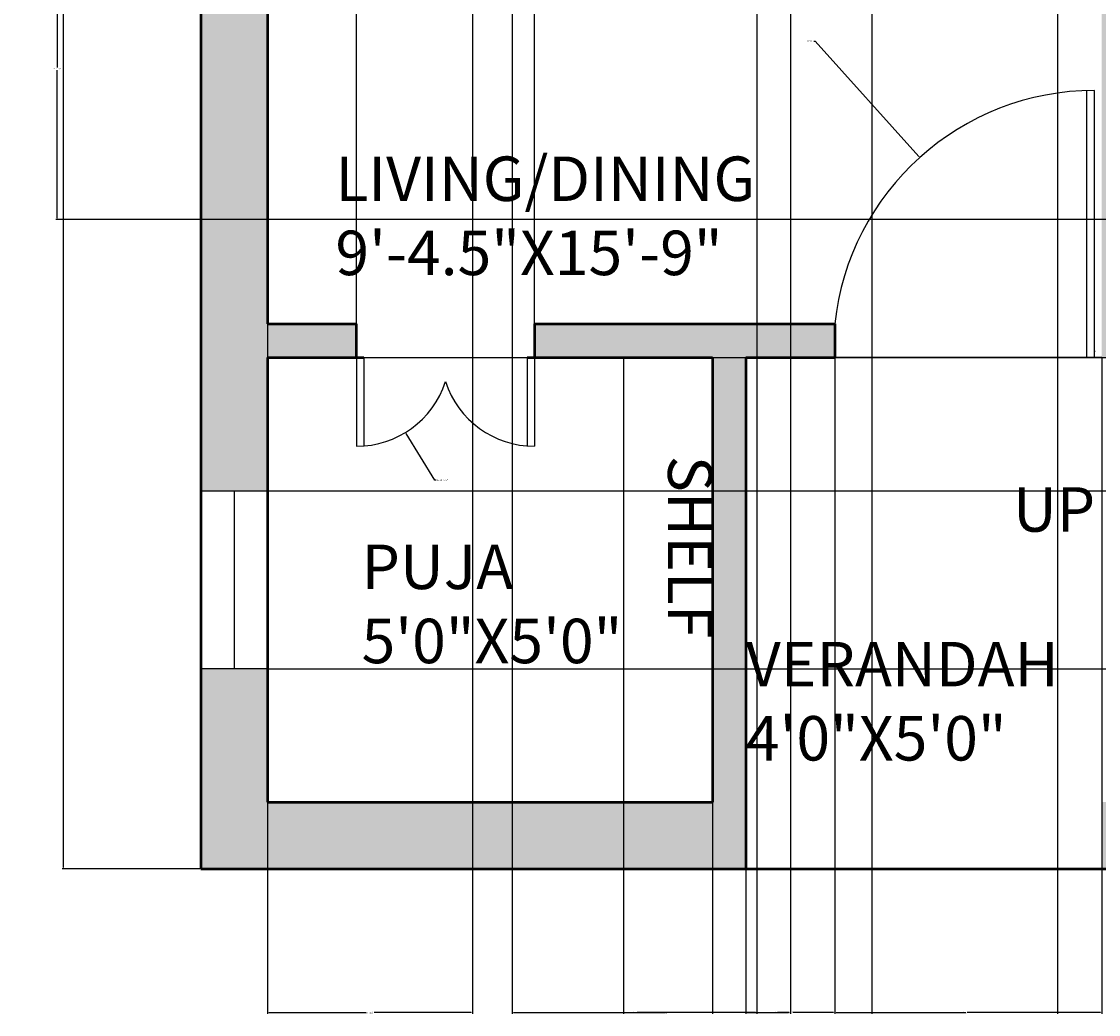
# Model space of a CAD drawing. Units: inches. Extents: x -2 to 282, y -370 to 35.
# Tile 1 of 5: x -2 to 143, y -370 to -237. Entities that reach past the tile are written whole.
import ezdxf

# ---------------------------------------------------------------- set-up
doc = ezdxf.new("R2010")
doc.units = ezdxf.units.IN
doc.header["$MEASUREMENT"] = 0
for name, color, linetype, lineweight in [('A-ANNO-DIMS', 2, 'Continuous', 18), ('A-ANNO-TEXT', 7, 'Continuous', 18), ('A-AREA-IDEN', 7, 'Continuous', 25), ('A-DOOR', 3, 'Continuous', 25), ('A-FLOR-CASE', 8, 'Continuous', 25), ('A-GLAZ', 4, 'Continuous', 25), ('A-WALL', 7, 'Continuous', 50), ('A-WALL-PATT', 252, 'Continuous', 13)]:
    doc.layers.add(name, color=color, linetype=linetype, lineweight=lineweight)
doc.styles.get("Standard").update_dxf_attribs({"font": 'arial.ttf'})
doc.dimstyles.get("Standard").update_dxf_attribs({"dimtxt": 0.18, "dimasz": 0.18, "dimexe": 0.18, "dimexo": 0.0625, "dimgap": 0.09, "dimtad": 0, "dimtih": 1, "dimtoh": 1, "dimdec": 0, "dimzin": 0, "dimdsep": 46, "dimlunit": 3, "dimtxsty": 'Standard', "dimcen": 0.09, "dimadec": 0, "dimazin": 0, "dimtfac": 1, "dimtdec": 0, "dimtofl": 0, "dimtmove": 0, "dimatfit": 3, "dimfxl": 1, "dimtolj": 1, "dimtzin": 0, "dimarcsym": 0})

# ---------------------------------------------------------------- blocks, each defined once
blk = doc.blocks.new('*D2')
at = {"layer": 'A-ANNO-DIMS', "color": 0, "lineweight": -2, "transparency": 16777216}
for p, q in [((22.35, 9.19), (3.74, 9.19)), ((3.92, 9.01), (3.92, -167.65)), ((3.92, -350.63), (3.92, -173.97)), ((22.35, -350.81), (3.74, -350.81))]:
    blk.add_line(p, q, dxfattribs=at)
at = {"layer": 'A-ANNO-DIMS', "color": 0, "transparency": 16777216}
for points in [[(3.89, 9.01), (3.95, 9.01), (3.92, 9.19)], [(3.89, -350.63), (3.95, -350.63), (3.92, -350.81)]]:
    blk.add_solid(points, dxfattribs=at)
at = {"layer": 'Defpoints', "color": 0, "transparency": 16777216}
for p in [(3.92, 9.19), (22.41, 9.19), (22.41, -350.81)]:
    blk.add_point(p, dxfattribs=at)
at = {"layer": 'A-ANNO-DIMS', "color": 0, "transparency": 16777216, "insert": (3.92, -170.81), "char_height": 6, "attachment_point": 5}
blk.add_mtext("\\A1;30'", dxfattribs=at)
blk = doc.blocks.new('*D31')
at = {"layer": 'A-ANNO-DIMS', "color": 0, "lineweight": -2, "transparency": 16777216}
for p, q in [((31.48, -281.81), (281.97, -281.81)), ((281.79, -281.99), (281.79, -290.63)), ((281.79, -299.63), (281.79, -290.99)), ((31.48, -299.81), (281.97, -299.81))]:
    blk.add_line(p, q, dxfattribs=at)
at = {"layer": 'A-ANNO-DIMS', "color": 0, "transparency": 16777216}
for points in [[(281.76, -281.99), (281.82, -281.99), (281.79, -281.81)], [(281.76, -299.63), (281.82, -299.63), (281.79, -299.81)]]:
    blk.add_solid(points, dxfattribs=at)
at = {"layer": 'Defpoints', "color": 0, "transparency": 16777216}
for p in [(31.41, -281.81), (31.41, -299.81), (281.79, -299.81)]:
    blk.add_point(p, dxfattribs=at)
at = {"layer": 'A-ANNO-DIMS', "color": 0, "transparency": 16777216, "insert": (281.79, -290.81), "char_height": 0.18, "attachment_point": 5}
blk.add_mtext('\\A1;1\'-6"', dxfattribs=at)
blk = doc.blocks.new('*D32')
at = {"layer": 'A-ANNO-DIMS', "color": 0, "lineweight": -2, "transparency": 16777216}
for p, q in [((31.48, -299.81), (281.97, -299.81)), ((281.79, -299.99), (281.79, -311.63)), ((281.79, -323.63), (281.79, -311.99)), ((31.48, -323.81), (281.97, -323.81))]:
    blk.add_line(p, q, dxfattribs=at)
at = {"layer": 'A-ANNO-DIMS', "color": 0, "transparency": 16777216}
for points in [[(281.76, -299.99), (281.82, -299.99), (281.79, -299.81)], [(281.76, -323.63), (281.82, -323.63), (281.79, -323.81)]]:
    blk.add_solid(points, dxfattribs=at)
at = {"layer": 'Defpoints', "color": 0, "transparency": 16777216}
for p in [(31.41, -299.81), (31.41, -323.81), (281.79, -323.81)]:
    blk.add_point(p, dxfattribs=at)
at = {"layer": 'A-ANNO-DIMS', "color": 0, "transparency": 16777216, "insert": (281.79, -311.81), "char_height": 0.18, "attachment_point": 5}
blk.add_mtext('\\A1;2\'-0"', dxfattribs=at)
blk = doc.blocks.new('*D35')
at = {"layer": 'A-ANNO-DIMS', "color": 0, "lineweight": -2, "transparency": 16777216}
for p, q in [((95.91, -281.87), (95.91, -370.37)), ((107.91, -281.87), (107.91, -370.37)), ((96.09, -370.19), (101.59, -370.19)), ((107.73, -370.19), (102.23, -370.19))]:
    blk.add_line(p, q, dxfattribs=at)
at = {"layer": 'A-ANNO-DIMS', "color": 0, "transparency": 16777216}
for points in [[(96.09, -370.16), (96.09, -370.22), (95.91, -370.19)], [(107.73, -370.16), (107.73, -370.22), (107.91, -370.19)]]:
    blk.add_solid(points, dxfattribs=at)
at = {"layer": 'Defpoints', "color": 0, "transparency": 16777216}
for p in [(95.91, -281.81), (107.91, -281.81), (107.91, -370.19)]:
    blk.add_point(p, dxfattribs=at)
at = {"layer": 'A-ANNO-DIMS', "color": 0, "transparency": 16777216, "insert": (101.91, -370.19), "char_height": 0.18, "attachment_point": 5}
blk.add_mtext('\\A1;1\'-0"', dxfattribs=at)
blk = doc.blocks.new('*D36')
at = {"layer": 'A-ANNO-DIMS', "color": 0, "lineweight": -2, "transparency": 16777216}
for p, q in [((107.91, -281.87), (107.91, -370.37)), ((143.91, -281.87), (143.91, -370.37)), ((108.09, -370.19), (125.58, -370.19)), ((143.73, -370.19), (126.24, -370.19))]:
    blk.add_line(p, q, dxfattribs=at)
at = {"layer": 'A-ANNO-DIMS', "color": 0, "transparency": 16777216}
for points in [[(108.09, -370.16), (108.09, -370.22), (107.91, -370.19)], [(143.73, -370.16), (143.73, -370.22), (143.91, -370.19)]]:
    blk.add_solid(points, dxfattribs=at)
at = {"layer": 'Defpoints', "color": 0, "transparency": 16777216}
for p in [(107.91, -281.81), (143.91, -281.81), (143.91, -370.19)]:
    blk.add_point(p, dxfattribs=at)
at = {"layer": 'A-ANNO-DIMS', "color": 0, "transparency": 16777216, "insert": (125.91, -370.19), "char_height": 0.18, "attachment_point": 5}
blk.add_mtext('\\A1;3\'-0"', dxfattribs=at)
blk = doc.blocks.new('*D37')
at = {"layer": 'A-ANNO-DIMS', "color": 0, "lineweight": -2, "transparency": 16777216}
for p, q in [((31.41, -277.25), (31.41, 28.74)), ((31.59, 28.56), (37.09, 28.56)), ((43.23, 28.56), (37.73, 28.56)), ((43.41, -277.25), (43.41, 28.74))]:
    blk.add_line(p, q, dxfattribs=at)
at = {"layer": 'A-ANNO-DIMS', "color": 0, "transparency": 16777216}
for points in [[(31.59, 28.59), (31.59, 28.53), (31.41, 28.56)], [(43.23, 28.59), (43.23, 28.53), (43.41, 28.56)]]:
    blk.add_solid(points, dxfattribs=at)
at = {"layer": 'Defpoints', "color": 0, "transparency": 16777216}
for p in [(43.41, 28.56), (31.41, -277.31), (43.41, -277.31)]:
    blk.add_point(p, dxfattribs=at)
at = {"layer": 'A-ANNO-DIMS', "color": 0, "transparency": 16777216, "insert": (37.41, 28.56), "char_height": 0.18, "attachment_point": 5}
blk.add_mtext('\\A1;1\'-0"', dxfattribs=at)
blk = doc.blocks.new('*D38')
at = {"layer": 'A-ANNO-DIMS', "color": 0, "lineweight": -2, "transparency": 16777216}
for p, q in [((43.41, -277.25), (43.41, 28.74)), ((43.59, 28.56), (55.08, 28.56)), ((67.23, 28.56), (55.74, 28.56)), ((67.41, -277.25), (67.41, 28.74))]:
    blk.add_line(p, q, dxfattribs=at)
at = {"layer": 'A-ANNO-DIMS', "color": 0, "transparency": 16777216}
for points in [[(43.59, 28.59), (43.59, 28.53), (43.41, 28.56)], [(67.23, 28.59), (67.23, 28.53), (67.41, 28.56)]]:
    blk.add_solid(points, dxfattribs=at)
at = {"layer": 'Defpoints', "color": 0, "transparency": 16777216}
for p in [(67.41, 28.56), (43.41, -277.31), (67.41, -277.31)]:
    blk.add_point(p, dxfattribs=at)
at = {"layer": 'A-ANNO-DIMS', "color": 0, "transparency": 16777216, "insert": (55.41, 28.56), "char_height": 0.18, "attachment_point": 5}
blk.add_mtext('\\A1;2\'-0"', dxfattribs=at)
blk = doc.blocks.new('*D39')
at = {"layer": 'A-ANNO-DIMS', "color": 0, "lineweight": -2, "transparency": 16777216}
for p, q in [((64.41, -88.37), (64.41, -370.37)), ((97.41, -88.37), (97.41, -370.37)), ((64.59, -370.19), (80.58, -370.19)), ((97.23, -370.19), (81.24, -370.19))]:
    blk.add_line(p, q, dxfattribs=at)
at = {"layer": 'A-ANNO-DIMS', "color": 0, "transparency": 16777216}
for points in [[(64.59, -370.16), (64.59, -370.22), (64.41, -370.19)], [(97.23, -370.16), (97.23, -370.22), (97.41, -370.19)]]:
    blk.add_solid(points, dxfattribs=at)
at = {"layer": 'Defpoints', "color": 0, "transparency": 16777216}
for p in [(64.41, -88.31), (97.41, -88.31), (97.41, -370.19)]:
    blk.add_point(p, dxfattribs=at)
at = {"layer": 'A-ANNO-DIMS', "color": 0, "transparency": 16777216, "insert": (80.91, -370.19), "char_height": 0.18, "attachment_point": 5}
blk.add_mtext('\\A1;2\'-9"', dxfattribs=at)
blk = doc.blocks.new('*D42')
at = {"layer": 'A-ANNO-DIMS', "color": 0, "lineweight": -2, "transparency": 16777216}
for p, q in [((31.41, -83.87), (31.41, -370.37)), ((59.05, -83.87), (59.05, -370.37)), ((31.59, -370.19), (44.69, -370.19)), ((58.87, -370.19), (45.77, -370.19))]:
    blk.add_line(p, q, dxfattribs=at)
at = {"layer": 'A-ANNO-DIMS', "color": 0, "transparency": 16777216}
for points in [[(31.59, -370.16), (31.59, -370.22), (31.41, -370.19)], [(58.87, -370.16), (58.87, -370.22), (59.05, -370.19)]]:
    blk.add_solid(points, dxfattribs=at)
at = {"layer": 'Defpoints', "color": 0, "transparency": 16777216}
for p in [(31.41, -83.81), (59.05, -83.81), (59.05, -370.19)]:
    blk.add_point(p, dxfattribs=at)
at = {"layer": 'A-ANNO-DIMS', "color": 0, "transparency": 16777216, "insert": (45.23, -370.19), "char_height": 0.18, "attachment_point": 5}
blk.add_mtext('\\A1;2\'-3 1/2"', dxfattribs=at)
blk = doc.blocks.new('*D46')
at = {"layer": 'A-ANNO-DIMS', "color": 0, "lineweight": -2, "transparency": 16777216}
for p, q in [((97.41, -88.37), (97.41, -370.37)), ((101.91, -88.37), (101.91, -370.37)), ((97.59, -370.19), (99.12, -370.19)), ((101.73, -370.19), (100.2, -370.19))]:
    blk.add_line(p, q, dxfattribs=at)
at = {"layer": 'A-ANNO-DIMS', "color": 0, "transparency": 16777216}
for points in [[(97.59, -370.16), (97.59, -370.22), (97.41, -370.19)], [(101.73, -370.16), (101.73, -370.22), (101.91, -370.19)]]:
    blk.add_solid(points, dxfattribs=at)
at = {"layer": 'Defpoints', "color": 0, "transparency": 16777216}
for p in [(97.41, -88.31), (101.91, -88.31), (101.91, -370.19)]:
    blk.add_point(p, dxfattribs=at)
at = {"layer": 'A-ANNO-DIMS', "color": 0, "transparency": 16777216, "insert": (99.66, -370.19), "char_height": 0.18, "attachment_point": 5}
blk.add_mtext('\\A1;0\'-4 1/2"', dxfattribs=at)
blk = doc.blocks.new('*D47')
at = {"layer": 'A-ANNO-DIMS', "color": 0, "lineweight": -2, "transparency": 16777216}
for p, q in [((79.41, -341.87), (79.41, -370.37)), ((91.41, -341.87), (91.41, -370.37)), ((79.59, -370.19), (85.09, -370.19)), ((91.23, -370.19), (85.73, -370.19))]:
    blk.add_line(p, q, dxfattribs=at)
at = {"layer": 'A-ANNO-DIMS', "color": 0, "transparency": 16777216}
for points in [[(79.59, -370.16), (79.59, -370.22), (79.41, -370.19)], [(91.23, -370.16), (91.23, -370.22), (91.41, -370.19)]]:
    blk.add_solid(points, dxfattribs=at)
at = {"layer": 'Defpoints', "color": 0, "transparency": 16777216}
for p in [(79.41, -341.81), (91.41, -341.81), (91.41, -370.19)]:
    blk.add_point(p, dxfattribs=at)
at = {"layer": 'A-ANNO-DIMS', "color": 0, "transparency": 16777216, "insert": (85.41, -370.19), "char_height": 0.18, "attachment_point": 5}
blk.add_mtext('\\A1;1\'-0"', dxfattribs=at)
blk = doc.blocks.new('*D48')
at = {"layer": 'A-ANNO-DIMS', "color": 0, "lineweight": -2, "transparency": 16777216}
for p, q in [((112.88, -229.72), (112.88, -370.37)), ((137.95, -229.72), (137.95, -370.37)), ((113.06, -370.19), (125.08, -370.19)), ((137.77, -370.19), (125.74, -370.19))]:
    blk.add_line(p, q, dxfattribs=at)
at = {"layer": 'A-ANNO-DIMS', "color": 0, "transparency": 16777216}
for points in [[(113.06, -370.16), (113.06, -370.22), (112.88, -370.19)], [(137.77, -370.16), (137.77, -370.22), (137.95, -370.19)]]:
    blk.add_solid(points, dxfattribs=at)
at = {"layer": 'Defpoints', "color": 0, "transparency": 16777216}
for p in [(112.88, -229.66), (137.95, -229.66), (137.95, -370.19)]:
    blk.add_point(p, dxfattribs=at)
at = {"layer": 'A-ANNO-DIMS', "color": 0, "transparency": 16777216, "insert": (125.41, -370.19), "char_height": 0.18, "attachment_point": 5}
blk.add_mtext('\\A1;2\'-1"', dxfattribs=at)
blk = doc.blocks.new('*D53')
at = {"layer": 'A-ANNO-DIMS', "color": 0, "lineweight": -2, "transparency": 16777216}
for p, q in [((185.51, -222.58), (2.86, -222.58)), ((3.04, -222.76), (3.04, -242.71)), ((3.04, -263.02), (3.04, -243.07)), ((185.51, -263.2), (2.86, -263.2))]:
    blk.add_line(p, q, dxfattribs=at)
at = {"layer": 'A-ANNO-DIMS', "color": 0, "transparency": 16777216}
for points in [[(3.01, -222.76), (3.07, -222.76), (3.04, -222.58)], [(3.01, -263.02), (3.07, -263.02), (3.04, -263.2)]]:
    blk.add_solid(points, dxfattribs=at)
at = {"layer": 'Defpoints', "color": 0, "transparency": 16777216}
for p in [(3.04, -222.58), (185.58, -222.58), (185.58, -263.2)]:
    blk.add_point(p, dxfattribs=at)
at = {"layer": 'A-ANNO-DIMS', "color": 0, "transparency": 16777216, "insert": (3.04, -242.89), "char_height": 0.18, "attachment_point": 5}
blk.add_mtext('\\A1;3\'-4 1/2"', dxfattribs=at)
blk = doc.blocks.new('*D62')
at = {"layer": 'A-ANNO-DIMS', "color": 0, "lineweight": -2, "transparency": 16777216}
for p, q in [((105.06, -239.15), (105.24, -239.15)), ((105.24, -239.15), (119.25, -254.71)), ((142.82, -281), (143, -281)), ((142.91, -281.09), (142.91, -280.91))]:
    blk.add_line(p, q, dxfattribs=at)
at = {"layer": 'A-ANNO-DIMS', "color": 0, "transparency": 16777216}
blk.add_solid([(119.27, -254.69), (119.23, -254.73), (119.37, -254.84)], dxfattribs=at)
at = {"layer": 'Defpoints', "color": 0, "transparency": 16777216}
for p in [(119.37, -254.84), (142.91, -281)]:
    blk.add_point(p, dxfattribs=at)
at = {"layer": 'A-ANNO-DIMS', "color": 0, "transparency": 16777216, "insert": (104.58, -239.15), "char_height": 0.18, "attachment_point": 5}
blk.add_mtext('\\A1;R2\'-11"', dxfattribs=at)
blk = doc.blocks.new('*D63')
at = {"layer": 'A-ANNO-DIMS', "color": 0, "lineweight": -2, "transparency": 16777216}
for p, q in [((43.32, -281.2), (43.5, -281.2)), ((43.41, -281.29), (43.41, -281.11)), ((53.99, -298.38), (50.12, -292.09)), ((54.17, -298.38), (53.99, -298.38))]:
    blk.add_line(p, q, dxfattribs=at)
at = {"layer": 'A-ANNO-DIMS', "color": 0, "transparency": 16777216}
blk.add_solid([(50.14, -292.08), (50.09, -292.11), (50.02, -291.94)], dxfattribs=at)
at = {"layer": 'Defpoints', "color": 0, "transparency": 16777216}
for p in [(43.41, -281.2), (50.02, -291.94)]:
    blk.add_point(p, dxfattribs=at)
at = {"layer": 'A-ANNO-DIMS', "color": 0, "transparency": 16777216, "insert": (54.99, -298.38), "char_height": 0.18, "attachment_point": 5}
blk.add_mtext('\\A1;2X R1\'-0 1/2"', dxfattribs=at)

msp = doc.modelspace()

# ---------------------------------------------------------------- hatches: boundary and pattern name
at = {"layer": 'A-WALL-PATT'}
h = msp.add_hatch(color=256, dxfattribs=at)
h.dxf.hatch_style = 1
h.paths.add_polyline_path([(262.41, 9.19), (134.91, 9.19), (134.91, 0.19), (143.91, 0.19), (143.91, -35.81), (148.41, -35.81), (148.41, 0.19), (253.41, 0.19), (253.41, -29.06), (262.41, -29.06)])
h.paths.add_polyline_path([(110.91, 9.19), (22.41, 9.19), (22.41, -11.81), (31.41, -11.81), (31.41, 0.19), (97.41, 0.19), (97.41, -88.31), (101.91, -88.31), (101.91, -64.31), (143.91, -64.31), (143.91, -88.31), (148.41, -88.31), (148.41, -59.81), (101.91, -59.81), (101.91, 0.19), (110.91, 0.19)])
h.paths.add_polyline_path([(31.41, -88.31), (64.41, -88.31), (64.41, -83.81), (31.41, -83.81), (31.41, -71.81), (22.41, -71.81), (22.41, -121.2), (31.41, -121.2)])
h.paths.add_polyline_path([(262.41, -89.06), (253.41, -89.06), (253.41, -118.31), (143.91, -118.31), (143.91, -122.81), (184.41, -122.81), (184.41, -164.81), (184.41, -169.31), (188.91, -169.31), (188.91, -164.81), (188.91, -122.81), (253.41, -122.81), (253.41, -131.81), (262.41, -131.81)])
h.paths.add_polyline_path([(262.41, -155.81), (253.41, -155.81), (253.41, -164.81), (212.91, -164.81), (212.91, -169.31), (253.41, -169.31), (253.41, -193.31), (262.41, -193.31)])
h.paths.add_polyline_path([(262.41, -253.31), (253.41, -253.31), (253.41, -277.31), (148.41, -277.31), (148.41, -164.81), (143.91, -164.81), (143.91, -169.31), (143.91, -281.81), (253.41, -281.81), (253.41, -341.81), (143.91, -341.81), (143.91, -350.81), (262.41, -350.81)])
h.paths.add_polyline_path([(31.41, -323.81), (22.41, -323.81), (22.41, -350.81), (95.91, -350.81), (95.91, -281.81), (107.91, -281.81), (107.91, -277.31), (67.41, -277.31), (67.41, -281.81), (91.41, -281.81), (91.41, -341.81), (31.41, -341.81)])
h.paths.add_polyline_path([(43.41, -277.31), (31.41, -277.31), (31.41, -181.2), (22.41, -181.2), (22.41, -299.81), (31.41, -299.81), (31.41, -281.81), (43.41, -281.81)])

# ---------------------------------------------------------------- linework, layer by layer
at = {"layer": 'A-DOOR'}
for p, q in [((141.91, -281.81), (141.91, -245.81)), ((142.91, -281.81), (142.91, -245.81)), ((43.41, -281.81), (43.41, -293.81)), ((44.41, -281.81), (44.41, -293.81)), ((66.41, -281.81), (66.41, -293.81)), ((67.41, -281.81), (67.41, -293.81)), ((142.91, -281.81), (107.91, -281.81)), ((143.91, -281.81), (142.91, -281.81))]:
    msp.add_line(p, q, dxfattribs=at)
for centre, radius, start, end in [((142.91, -281), 35.19, 90, 173.9744), ((43.41, -281.2), 12.61, 270, 342.0547), ((67.41, -281.2), 12.61, 197.9453, 270)]:
    msp.add_arc(centre, radius, start, end, dxfattribs=at)
at = {"layer": 'A-FLOR-CASE'}
msp.add_line((79.41, -281.81), (79.41, -341.81), dxfattribs=at)
at = {"layer": 'A-GLAZ'}
for p, q in [((22.41, -323.81), (22.41, -299.81)), ((22.41, -299.81), (31.41, -299.81)), ((26.91, -299.81), (26.91, -323.81)), ((31.41, -299.81), (31.41, -323.81)), ((31.41, -323.81), (22.41, -323.81))]:
    msp.add_line(p, q, dxfattribs=at)
at = {"layer": 'A-WALL'}
for p, q in [((22.41, 9.19), (22.41, -350.81)), ((31.41, -88.31), (31.41, -277.31)), ((31.41, -277.31), (43.41, -277.31)), ((43.41, -281.81), (43.41, -277.31)), ((67.41, -277.31), (67.41, -281.81)), ((67.41, -277.31), (107.91, -277.31)), ((107.91, -277.31), (107.91, -281.81)), ((31.41, -281.81), (44.41, -281.81)), ((31.41, -281.81), (31.41, -341.81)), ((66.41, -281.81), (91.41, -281.81)), ((91.41, -281.81), (91.41, -341.81)), ((95.91, -281.81), (95.91, -350.81)), ((95.91, -281.81), (107.91, -281.81)), ((31.41, -341.81), (91.41, -341.81)), ((22.41, -350.81), (262.41, -350.81))]:
    msp.add_line(p, q, dxfattribs=at)

# ---------------------------------------------------------------- texts
at = {"layer": 'A-ANNO-TEXT', "insert": (91.41, -295.09), "char_height": 6, "attachment_point": 1, "rotation": 270}
msp.add_mtext_dynamic_manual_height_columns('SHELF', width=3.1748, gutter_width=1, heights=[0], dxfattribs=at)
at = {"layer": 'A-ANNO-TEXT', "insert": (131.93, -299.33), "char_height": 6, "attachment_point": 1}
msp.add_mtext('UP', dxfattribs=at)
at = {"layer": 'A-AREA-IDEN', "char_height": 6, "attachment_point": 1}
for s, insert in [('LIVING/DINING\\P9\'-4.5"X15\'-9"', (40.56, -254.72)), ('PUJA\\P5\'0"X5\'0"', (44.09, -307.07)), ('VERANDAH\\P4\'0"X5\'0"', (95.91, -320.2))]:
    msp.add_mtext(s, dxfattribs=dict(at, insert=insert))

# ---------------------------------------------------------------- dimensions: what is measured, and where the dimension line sits
at = {"layer": 'A-ANNO-DIMS'}
for base, p1, p2, picture, middle in [((43.41, 28.56), (31.41, -277.31), (43.41, -277.31), '*D37', (37.41, 28.56)), ((67.41, 28.56), (43.41, -277.31), (67.41, -277.31), '*D38', (55.41, 28.56)), ((59.05, -370.19), (31.41, -83.81), (59.05, -83.81), '*D42', (45.23, -370.19)), ((97.41, -370.19), (64.41, -88.31), (97.41, -88.31), '*D39', (80.91, -370.19)), ((101.91, -370.19), (97.41, -88.31), (101.91, -88.31), '*D46', (99.66, -370.19)), ((137.95, -370.19), (112.88, -229.66), (137.95, -229.66), '*D48', (125.41, -370.19)), ((107.91, -370.19), (95.91, -281.81), (107.91, -281.81), '*D35', (101.91, -370.19)), ((143.91, -370.19), (107.91, -281.81), (143.91, -281.81), '*D36', (125.91, -370.19)), ((91.41, -370.19), (79.41, -341.81), (91.41, -341.81), '*D47', (85.41, -370.19))]:
    dim = msp.add_linear_dim(base=base, p1=p1, p2=p2, dimstyle='Standard', override={"dimdec": 1, "dimlfac": 1, "dimrnd": 0, "dimzin": 1, "dimdsep": 46, "dimlunit": 4, "dimfrac": 2}, dxfattribs=at)
    dim.commit()
    dim.dimension.update_dxf_attribs({"geometry": picture, "text_midpoint": middle})
for base, p1, p2, override, picture, middle in [((3.92, 9.19), (22.41, -350.81), (22.41, 9.19), {"dimtxt": 6, "dimclrd": 0, "dimclre": 0, "dimclrt": 0}, '*D2', (3.92, -170.81)), ((3.04, -222.58), (185.58, -263.2), (185.58, -222.58), {"dimdec": 1, "dimlfac": 1, "dimrnd": 0, "dimzin": 1, "dimdsep": 46, "dimlunit": 4, "dimfrac": 2}, '*D53', (3.04, -242.89)), ((281.79, -299.81), (31.41, -281.81), (31.41, -299.81), {"dimdec": 1, "dimlfac": 1, "dimrnd": 0, "dimzin": 1, "dimdsep": 46, "dimlunit": 4, "dimfrac": 2}, '*D31', (281.79, -290.81)), ((281.79, -323.81), (31.41, -299.81), (31.41, -323.81), {"dimdec": 1, "dimlfac": 1, "dimrnd": 0, "dimzin": 1, "dimdsep": 46, "dimlunit": 4, "dimfrac": 2}, '*D32', (281.79, -311.81))]:
    dim = msp.add_linear_dim(base=base, p1=p1, p2=p2, angle=90, dimstyle='Standard', override=override, dxfattribs=at)
    dim.commit()
    dim.dimension.update_dxf_attribs({"geometry": picture, "text_midpoint": middle})
dim = msp.add_radius_dim(center=(142.91, -281), mpoint=(119.37, -254.84), dimstyle='Standard', override={"dimdec": 1, "dimlfac": 1, "dimrnd": 0, "dimzin": 1, "dimdsep": 46, "dimlunit": 4, "dimfrac": 2}, dxfattribs=at)
dim.commit()
dim.dimension.update_dxf_attribs({"geometry": '*D62', "text_midpoint": (104.58, -239.15), "dimtype": 164})
dim = msp.add_radius_dim(center=(43.41, -281.2), mpoint=(50.02, -291.94), text='2X <>', dimstyle='Standard', override={"dimdec": 1, "dimlfac": 1, "dimrnd": 0, "dimzin": 1, "dimdsep": 46, "dimlunit": 4, "dimfrac": 2}, dxfattribs=at)
dim.commit()
dim.dimension.update_dxf_attribs({"geometry": '*D63', "text_midpoint": (54.99, -298.38), "dimtype": 164})

doc.saveas('drawing.dxf')
